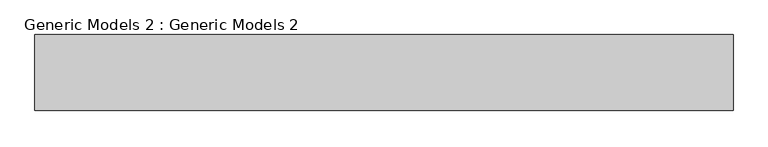
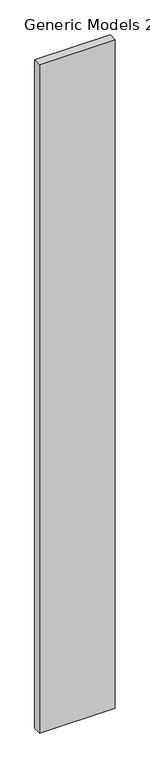
"""IFC4 building model written with IfcOpenShell, lengths in millimetres: proxy geometry, Generic Models 2 : Generic Models 2."""

from ifc_helpers import new_model, si_unit, origin, place, context, project, spatial, faceted_brep, source, transform, mapped, element, save


def generic_models_2_generic_models_2_1119aa77(model_context):
    return source(origin(), model_context, "Body", "Brep", [
        faceted_brep([(-17832.2537599, -14261.7752569, -228.6), (-17832.2537599, -14261.7752569, 9321.8), (-17832.2537599, -14261.7752569, 10663.5282636), (-18997.6195233, -14261.7752569, 10663.5282636), (-18997.6195233, -14261.7752569, -228.6), (-17832.2537599, -14134.7752569, -228.6), (-18997.6195233, -14134.7752569, -228.6), (-18997.6195233, -14134.7752569, 10663.5282636), (-17832.2537599, -14134.7752569, 10663.5282636), (-17832.2537599, -14134.7752569, 9321.8)], [[[0, 1, 2, 3, 4]], [[5, 6, 7, 8, 9]], [[2, 1, 0, 5, 9, 8]], [[3, 2, 8, 7]], [[4, 3, 7, 6]], [[0, 4, 6, 5]]]),
    ])


if __name__ == "__main__":
    model = new_model("IFC4")
    model_context = context("Model", 3, world=origin())
    ifc_project = project(units=[si_unit("LENGTHUNIT", "METRE", prefix="MILLI")], contexts=[model_context])
    site = spatial("IfcSite", under=ifc_project)
    building = spatial("IfcBuilding", under=site)
    placement = place(None, origin())
    generic_models_2_generic_models_2_shape = generic_models_2_generic_models_2_1119aa77(model_context)
    element("IfcBuildingElementProxy", 1, Name="Generic Models 2 : Generic Models 2", ObjectType="Generic Models 2 : Generic Models 2", at=placement, inside=building, context=model_context, shape_type="MappedRepresentation", body=[
        mapped(generic_models_2_generic_models_2_shape, transform((0.0, 0.0, 0.0), x_axis=(1.0, 0.0, 0.0), y_axis=(0.0, 1.0, 0.0), z_axis=(0.0, 0.0, 1.0))),
    ])
    save(model, "model.ifc")
